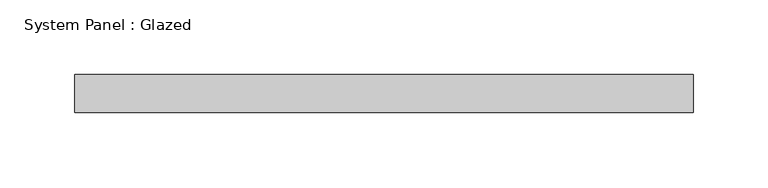
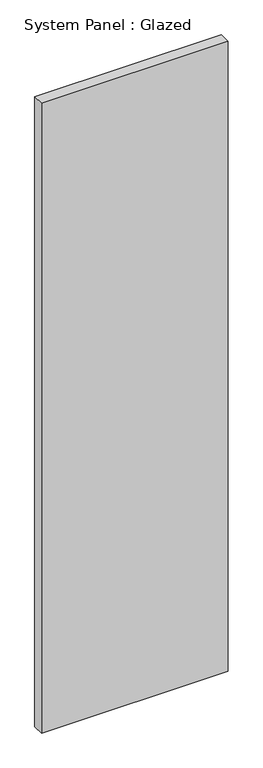
"""IFC4 building model written with IfcOpenShell, lengths in millimetres: plate geometry, System Panel : Glazed."""

from ifc_helpers import new_model, si_unit, origin, origin_with_axes, place, context, project, spatial, polyline, outline, extrude, source, transform, mapped, element, save


def system_panel_glazed_02e859a2(model_context):
    return source(origin(), model_context, "Body", "SweptSolid", [
        extrude(outline(polyline([(206.375, 19.05), (-206.375, 19.05), (-206.375, 44.45), (206.375, 44.45), (206.375, 19.05)])), origin_with_axes(), (0.0, 0.0, 1.0), 1472.5620987),
    ])


if __name__ == "__main__":
    model = new_model("IFC4")
    model_context = context("Model", 3, world=origin())
    ifc_project = project(units=[si_unit("LENGTHUNIT", "METRE", prefix="MILLI")], contexts=[model_context])
    site = spatial("IfcSite", under=ifc_project)
    building = spatial("IfcBuilding", under=site)
    placement = place(None, origin())
    system_panel_glazed_shape = system_panel_glazed_02e859a2(model_context)
    element("IfcPlate", 1, ObjectType="System Panel : Glazed", at=placement, inside=building, context=model_context, shape_type="MappedRepresentation", body=[
        mapped(system_panel_glazed_shape, transform((0.0, 0.0, 0.0), x_axis=(1.0, 0.0, 0.0), y_axis=(0.0, 1.0, 0.0), z_axis=(0.0, 0.0, 1.0))),
    ])
    save(model, "model.ifc")

# Revit data of these elements
# Type "System Panel : Glazed"
#   Construction Type Id = "GSP4R"
#   Analytic Construction = "1/8 in Pilkington single glazing"
#   Visual Light Transmittance = 0.9
#   Solar Heat Gain Coefficient = 0.86
#   Heat Transfer Coefficient (U) = 1.18115 BTU/(h·ft²·°F)
#   Define Thermal Properties by = 1
# Element 1 (IfcPlate, "System Panel : Glazed")
#   Materials on its faces: "Glass"
# Materials
#   "Glass": class "Glass", colour RGB 0 128 192, transparency 0.75, Description = "Soda Lime Glass", Cost = 0
